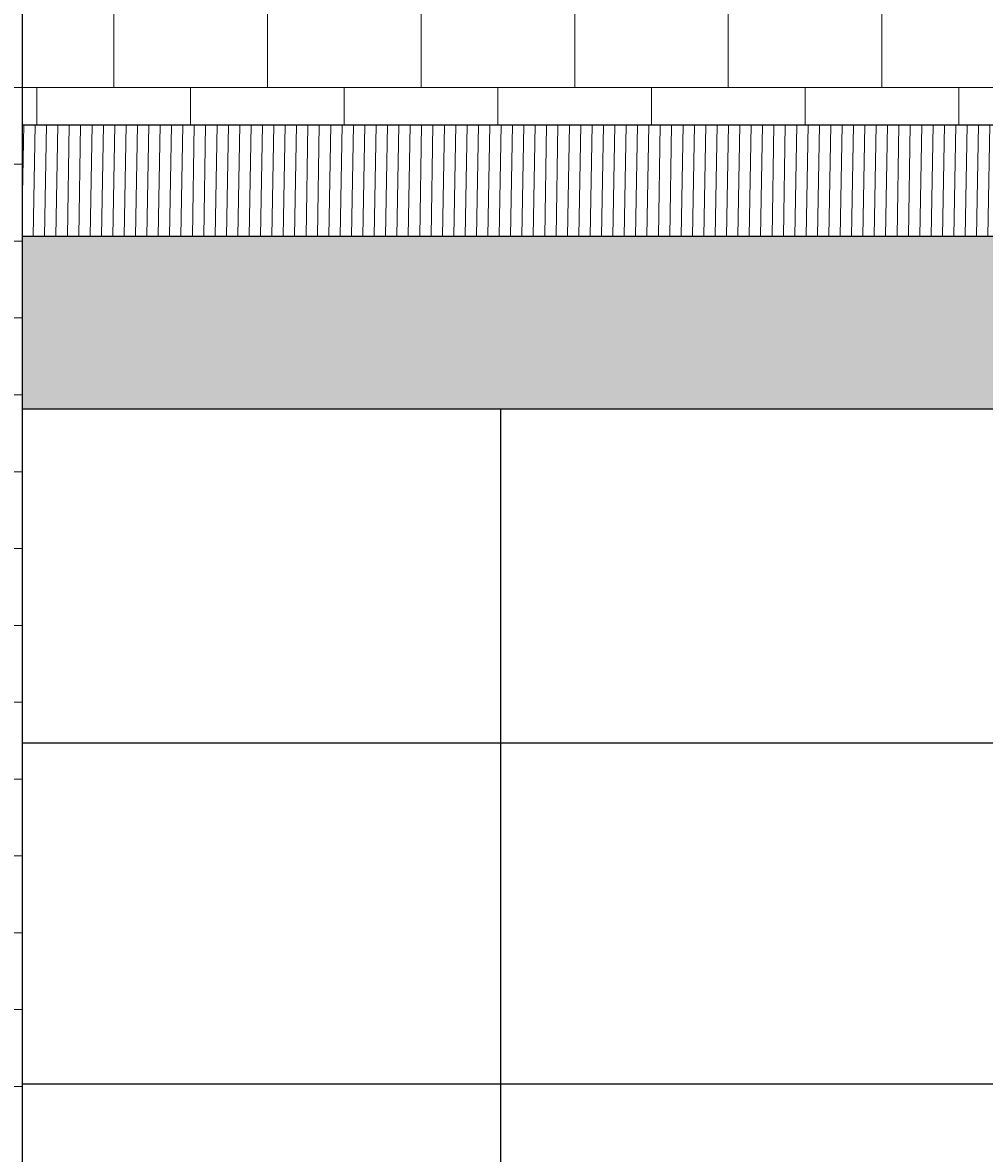
# Model space of a CAD drawing. Units: inches. Extents: x -26 to 776, y -22 to 650.
# Tile 4 of 62: x 23 to 98, y 67 to 155. Entities that reach past the tile are written whole.
import ezdxf

# ---------------------------------------------------------------- set-up
doc = ezdxf.new("R2010")
doc.units = ezdxf.units.IN
doc.header["$MEASUREMENT"] = 0
for name, color, linetype, lineweight in [('A-ANNO-DIMS', 2, 'Continuous', 18), ('A-DETL-PATT', 8, 'Continuous', 13), ('A-DOOR', 3, 'Continuous', 25), ('A-DOOR-PATT', 8, 'Continuous', 13), ('A-WALL-PATT', 8, 'Continuous', 13)]:
    doc.layers.add(name, color=color, linetype=linetype, lineweight=lineweight)
doc.styles.get("Standard").update_dxf_attribs({"font": 'arial.ttf'})
doc.dimstyles.get("Standard").update_dxf_attribs({"dimtxt": 0.5625, "dimasz": 0.18, "dimexe": 0.18, "dimexo": 0.0625, "dimgap": 0.09, "dimtad": 0, "dimtih": 1, "dimtoh": 1, "dimdec": 4, "dimzin": 0, "dimdsep": 46, "dimlunit": 4, "dimtxsty": 'Standard', "dimcen": 0.09, "dimadec": 0, "dimazin": 0, "dimtfac": 1, "dimtdec": 4, "dimtofl": 0, "dimtmove": 0, "dimatfit": 3, "dimfxl": 1, "dimtolj": 1, "dimtzin": 0, "dimarcsym": 0})

# ---------------------------------------------------------------- blocks, each defined once
blk = doc.blocks.new('*D14')
at = {"layer": 'A-ANNO-DIMS', "color": 0, "lineweight": -2, "transparency": 16777216}
for p, q in [((191.616, 613.271), (-25.478, 613.271)), ((-25.298, 613.091), (-25.298, 314.754)), ((-25.298, 15.662), (-25.298, 314)), ((11.045, 15.482), (-25.478, 15.482))]:
    blk.add_line(p, q, dxfattribs=at)
at = {"layer": 'A-ANNO-DIMS', "color": 0, "transparency": 16777216}
for points in [[(-25.328, 613.091), (-25.268, 613.091), (-25.298, 613.271)], [(-25.328, 15.662), (-25.268, 15.662), (-25.298, 15.482)]]:
    blk.add_solid(points, dxfattribs=at)
at = {"layer": 'Defpoints', "color": 0, "transparency": 16777216}
for p in [(-25.298, 613.271), (191.678, 613.271), (11.107, 15.482)]:
    blk.add_point(p, dxfattribs=at)
at = {"layer": 'A-ANNO-DIMS', "color": 0, "transparency": 16777216, "insert": (-25.298, 314.377), "char_height": 0.5625, "attachment_point": 5}
blk.add_mtext('\\A1;597.8', dxfattribs=at)
blk = doc.blocks.new('*D22')
at = {"layer": 'A-ANNO-DIMS', "color": 0, "lineweight": -2, "transparency": 16777216}
for p, q in [((22.889, 15.333), (22.889, 649.856)), ((217.953, 15.545), (217.953, 649.856)), ((23.069, 649.676), (119.19, 649.676)), ((217.773, 649.676), (121.652, 649.676))]:
    blk.add_line(p, q, dxfattribs=at)
at = {"layer": 'A-ANNO-DIMS', "color": 0, "transparency": 16777216}
for points in [[(23.069, 649.706), (23.069, 649.646), (22.889, 649.676)], [(217.773, 649.706), (217.773, 649.646), (217.953, 649.676)]]:
    blk.add_solid(points, dxfattribs=at)
at = {"layer": 'Defpoints', "color": 0, "transparency": 16777216}
for p in [(217.953, 649.676), (22.889, 15.27), (217.953, 15.482)]:
    blk.add_point(p, dxfattribs=at)
at = {"layer": 'A-ANNO-DIMS', "color": 0, "transparency": 16777216, "insert": (120.421, 649.676), "char_height": 0.5625, "attachment_point": 5}
blk.add_mtext('\\A1;195.06', dxfattribs=at)
blk = doc.blocks.new('*D37')
at = {"layer": 'A-ANNO-DIMS', "color": 0, "lineweight": -2, "transparency": 16777216}
for p, q in [((231.362, 159.482), (-25.478, 159.482)), ((-25.298, 159.302), (-25.298, 87.855)), ((-25.298, 15.662), (-25.298, 87.11)), ((217.89, 15.482), (-25.478, 15.482))]:
    blk.add_line(p, q, dxfattribs=at)
at = {"layer": 'A-ANNO-DIMS', "color": 0, "transparency": 16777216}
for points in [[(-25.328, 159.302), (-25.268, 159.302), (-25.298, 159.482)], [(-25.328, 15.662), (-25.268, 15.662), (-25.298, 15.482)]]:
    blk.add_solid(points, dxfattribs=at)
at = {"layer": 'Defpoints', "color": 0, "transparency": 16777216}
for p in [(-25.298, 159.482), (231.425, 159.482), (217.953, 15.482)]:
    blk.add_point(p, dxfattribs=at)
at = {"layer": 'A-ANNO-DIMS', "color": 0, "transparency": 16777216, "insert": (-25.298, 87.482), "char_height": 0.5625, "attachment_point": 5}
blk.add_mtext('\\A1;144', dxfattribs=at)

msp = doc.modelspace()

# ---------------------------------------------------------------- hatches: boundary and pattern name
at = {"layer": 'A-DETL-PATT'}
h = msp.add_hatch(dxfattribs=at)
h.set_pattern_fill('ANSI31', color=256, scale=7.1, angle=44)
h.paths.add_polyline_path([(231.4249, 197.3298), (216.1056, 197.3298), (216.1056, 159.4824), (231.4249, 159.4824)])
h.paths.add_polyline_path([(236.4647, 197.3298), (231.4249, 197.3298), (231.4249, 159.4824), (276.1134, 159.4824), (276.1134, 171.4173), (236.4647, 171.4173)])
h.paths.add_polyline_path([(259.7413, 197.3298), (236.4647, 197.3298), (236.4647, 171.4173), (259.7413, 171.4173)], flags=17)
h.paths.add_polyline_path([(276.1134, 197.3298), (261.7413, 197.3298), (261.7413, 171.4173), (276.1134, 171.4173)], flags=17)
h.paths.add_polyline_path([(217.9529, 147.0781), (22.8891, 147.0781), (22.8891, 138.3844), (217.9529, 138.3844)])
h.paths.add_polyline_path([(285.0179, 152.3087), (285.0179, 159.4824), (231.4249, 159.4824), (240.1654, 144.8359), (280.6173, 144.8359)])
h.paths.add_polyline_path([(280.6173, 144.8359), (240.1654, 144.8359), (240.1654, 26.4239), (280.6173, 26.4239)])
h.paths.add_polyline_path([(274.6644, 134.8811), (274.6644, 34.0885), (245.7207, 34.0885), (245.7207, 134.8811)], flags=16)
h.paths.add_polyline_path([(285.0179, 303.3046), (236.4647, 303.3046), (236.4647, 294.4171), (285.0179, 294.4171)])
h.paths.add_polyline_path([(285.0179, 446.0063), (236.4647, 446.0063), (236.4647, 437.1188), (285.0179, 437.1188)])
at = {"layer": 'A-DOOR-PATT'}
h = msp.add_hatch(color=256, dxfattribs=at)
h.dxf.hatch_style = 1
h.paths.add_polyline_path([(217.9529, 138.3844), (22.8891, 138.3844), (22.8891, 124.9232), (217.9529, 124.9232)])
h.paths.add_polyline_path([(274.6644, 134.8811), (245.7207, 134.8811), (245.7207, 34.0885), (274.6644, 34.0885)])
at = {"layer": 'A-WALL-PATT'}
h = msp.add_hatch(dxfattribs=at)
h.set_pattern_fill('AR-B816', color=256, scale=0.75)
h.paths.add_polyline_path([(82.134, 209.6413), (11.1074, 209.6413), (11.1074, 159.4824), (82.134, 159.4824)])
h.paths.add_polyline_path([(231.4249, 209.6413), (209.091, 209.6413), (209.091, 159.4824), (214.1056, 159.4824), (214.1056, 199.3298), (231.4249, 199.3298)])
h.paths.add_polyline_path([(231.4249, 159.4824), (11.1074, 159.4824), (11.1074, 22.5014), (22.8891, 22.5014), (22.8891, 147.0781), (217.9529, 147.0781), (217.9529, 20.7937), (231.4249, 20.7937)])
h.paths.add_polyline_path([(285.0179, 152.3087), (280.6173, 144.8359), (280.6173, 26.4239), (240.1654, 26.4239), (240.1654, 144.8359), (231.4249, 159.4824), (231.4249, 20.7937), (285.0179, 20.7937)])

# ---------------------------------------------------------------- linework, layer by layer
at = {"layer": 'A-DOOR'}
for p, q in [((22.8891, 15.2701), (22.8891, 147.0781)), ((22.8891, 147.0781), (217.9529, 147.0781)), ((22.8891, 138.3844), (217.9529, 138.3844)), ((22.8891, 124.9232), (217.9529, 124.9232)), ((60.2178, 124.9232), (60.2178, 15.4824)), ((22.8891, 98.842), (217.9529, 98.842)), ((22.8891, 72.2), (217.9529, 72.2))]:
    msp.add_line(p, q, dxfattribs=at)

# ---------------------------------------------------------------- dimensions: what is measured, and where the dimension line sits
at = {"layer": 'A-ANNO-DIMS'}
dim = msp.add_linear_dim(base=(217.9529, 649.6763), p1=(22.8891, 15.2701), p2=(217.9529, 15.4824), dimstyle='Standard', override={"dimdec": 2, "dimlfac": 1, "dimrnd": 0, "dimzin": 0, "dimdsep": 46, "dimlunit": 2}, dxfattribs=at)
dim.commit()
dim.dimension.update_dxf_attribs({"geometry": '*D22', "text_midpoint": (120.421, 649.6763)})
for base, p1, p2, override, picture, middle in [((-25.2976, 613.2713), (11.1074, 15.4824), (191.6782, 613.2713), {"dimdec": 1, "dimlfac": 1, "dimrnd": 0, "dimzin": 0, "dimdsep": 46, "dimlunit": 2}, '*D14', (-25.2976, 314.3769)), ((-25.2976, 159.4824), (217.9529, 15.4824), (231.4249, 159.4824), {"dimdec": 0, "dimlfac": 1, "dimrnd": 0, "dimzin": 0, "dimdsep": 46, "dimlunit": 2}, '*D37', (-25.2976, 87.4824))]:
    dim = msp.add_linear_dim(base=base, p1=p1, p2=p2, angle=90, dimstyle='Standard', override=override, dxfattribs=at)
    dim.commit()
    dim.dimension.update_dxf_attribs({"geometry": picture, "text_midpoint": middle})

doc.saveas('drawing.dxf')
